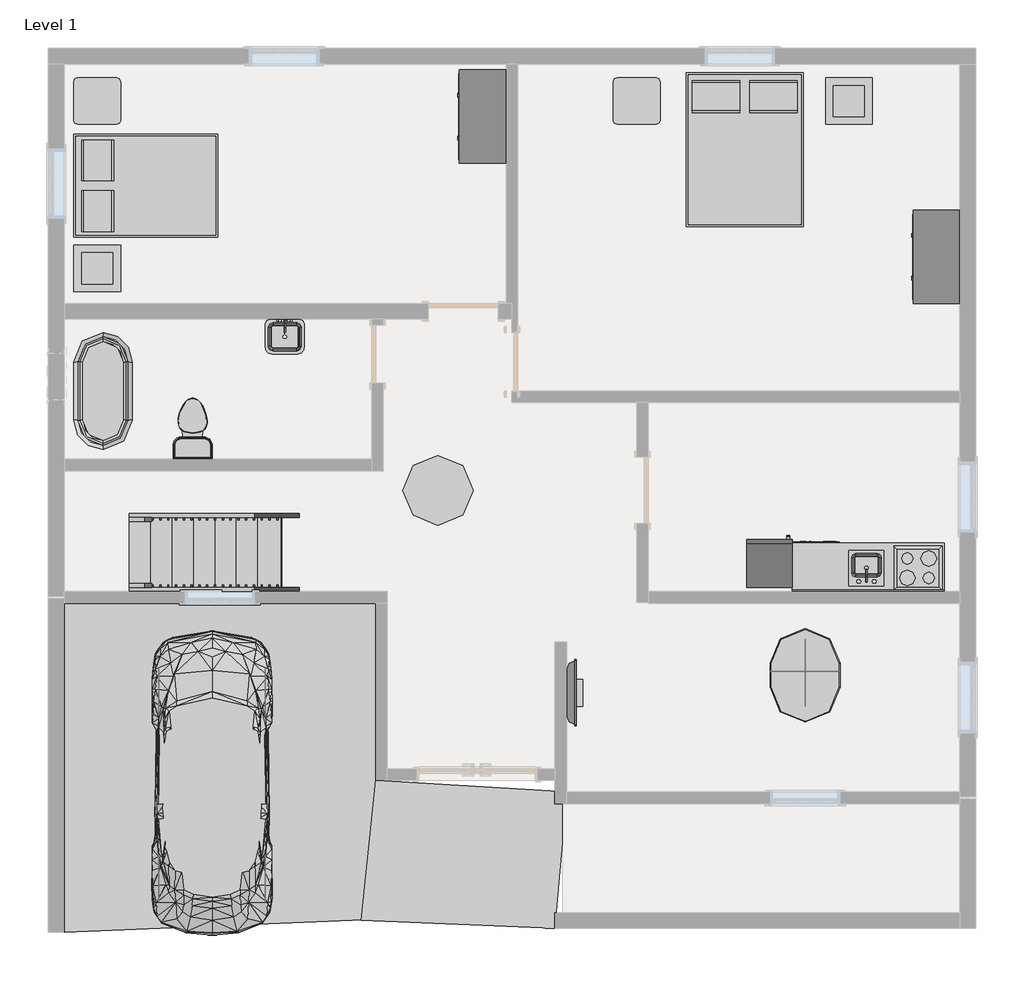
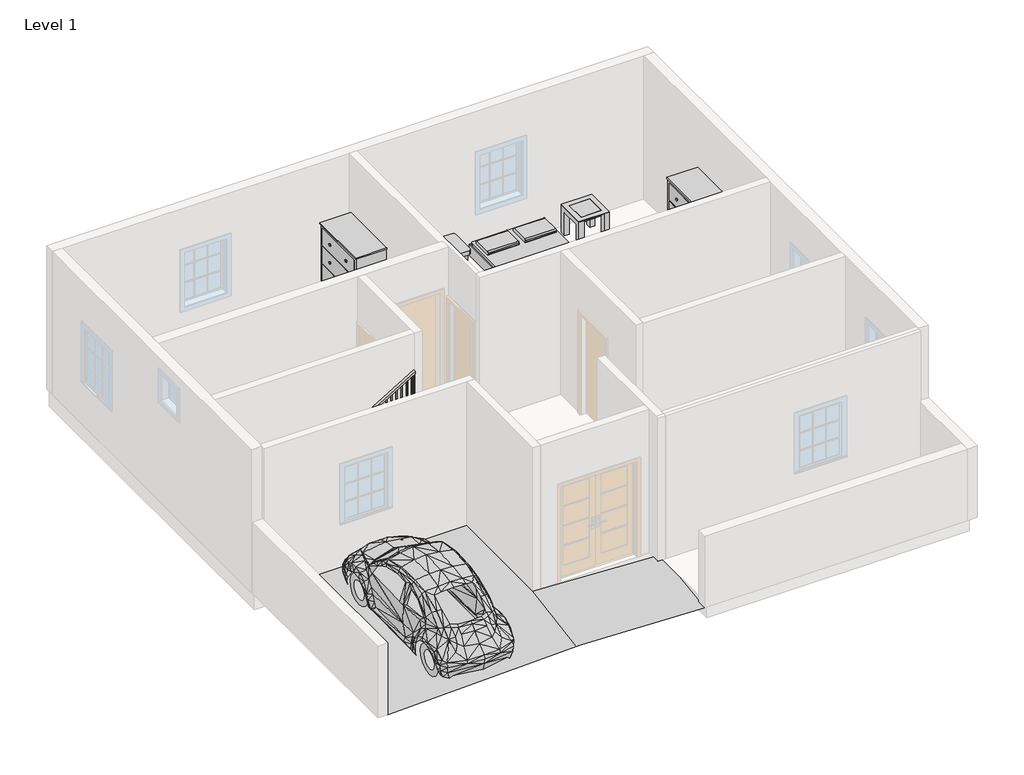
# One storey, part 2 of 2: 12 furniture elements, 7 proxies, 5 flow terminals, 2 members, 2 railings, 1 geographic element, 1 stair flight.
"""IFC4 building model written with IfcOpenShell, lengths in millimetres."""

from ifc_helpers import new_model, si_unit, frame, origin, place, context, project, spatial, polyline, outline, extrude, triangles, transform, mapped, element, save
from components import proxy_a6faaae8, proxy_45b28599, kitchenette_medium_kitchenette_medium_844211aa, rpc_beetle_rpc_beetle_3ce7ba48, proxy_c523a7b7, flow_terminal_2b63360b, flow_terminal_871c2e40, flow_terminal_62a433f7, toilet_domestic_3d_toilet_domestic_3d_f7549cf7, toilet_domestic_3d_toilet_domestic_3d_183bbd19, flow_terminal_b374fae2, furniture_c8abb964, furniture_1d2926bd, furniture_c6510c7c, furniture_9fa109b2, furniture_56245f3a, furniture_b5c51a22, furniture_be1c6672, furniture_905aceb5, furniture_bcf351fa, rpc_plant_tropical_agave_1_5_93a2a214, stair_flight_ef839ef7

model = new_model("IFC4")

# Units and contexts
model_context = context("Model", 3, world=origin())
ifc_project = project(units=[si_unit("LENGTHUNIT", "METRE", prefix="MILLI")], contexts=[model_context])

# Site, building, storey
site = spatial("IfcSite", under=ifc_project)
building = spatial("IfcBuilding", under=site)
storey = spatial("IfcBuildingStorey", under=building, Name="Level 1", Elevation=0.0)

# Proxies
placement = place(None, origin())
element("IfcBuildingElementProxy", 1, Name="Building Element Proxy", at=placement, inside=storey, context=model_context, shape_type="Tessellation", body=[
    triangles([(-9823.2573761, 4081.3729706, 0.0), (-7334.0575699, 3928.9729706, 0.0), (-7486.4575699, 2150.9729221, 0.0), (-9704.2471985, 2259.3859268, 0.0), (-10012.857431, 2253.2262737, 0.0)], [[1, 5, 4], [4, 3, 2], [3, 4, 5], [4, 2, 1]], closed=False),
])
element("IfcBuildingElementProxy", 2, Name="Building Element Proxy", at=placement, inside=storey, context=model_context, shape_type="Tessellation", body=[
    triangles([(-13887.2581512, 6392.7731644, 0.0), (-13887.2581512, 2100.1729706, 0.0), (-9823.2573761, 6392.7731644, 0.0), (-9969.6902985, 2259.3859268, 0.0), (-9823.2573761, 4081.3729706, 0.0)], [[1, 2, 5], [5, 3, 1], [5, 2, 4]], closed=False),
])
proxy_shape = proxy_a6faaae8(model_context)
element("IfcBuildingElementProxy", 3, Name="Cook Top-4 Unit2 : 22\" x 20\"", ObjectType="Cook Top-4 Unit2 : 22\" x 20\"", at=placement, inside=storey, context=model_context, shape_type="MappedRepresentation", body=[
    mapped(proxy_shape, transform((-2749.3576657, 6849.9729822, 0.0), x_axis=(-0.9999999999999998, 0.0, 0.0), y_axis=(0.0, -0.9999999999999998, 0.0), z_axis=(0.0, 0.0, 1.0))),
])
proxy_2_shape = proxy_45b28599(model_context)
element("IfcBuildingElementProxy", 4, Name="Dishwasher : 24\" x 24\" x 34\"", ObjectType="Dishwasher : 24\" x 24\" x 34\"", at=placement, inside=storey, context=model_context, shape_type="MappedRepresentation", body=[
    mapped(proxy_2_shape, transform((-3700.5401972, 7141.822547, 0.0), x_axis=(-0.9999999999999998, 0.0, 0.0), y_axis=(0.0, -0.9999999999999998, 0.0), z_axis=(0.0, 0.0, 1.0))),
])
kitchenette_medium_kitchenette_medium_shape = kitchenette_medium_kitchenette_medium_844211aa(model_context)
element("IfcBuildingElementProxy", 5, Name="Kitchenette - Medium : Kitchenette - Medium", ObjectType="Kitchenette - Medium : Kitchenette - Medium", at=placement, inside=storey, context=model_context, shape_type="MappedRepresentation", body=[
    mapped(kitchenette_medium_kitchenette_medium_shape, transform((-3073.5199608, 6545.1729822, 0.0), x_axis=(-0.9999999999999998, 0.0, 0.0), y_axis=(0.0, -0.9999999999999998, 0.0), z_axis=(0.0, 0.0, 1.0))),
])
rpc_beetle_rpc_beetle_shape = rpc_beetle_rpc_beetle_3ce7ba48(model_context)
element("IfcBuildingElementProxy", 6, Name="RPC Beetle : RPC Beetle", ObjectType="RPC Beetle : RPC Beetle", at=placement, inside=storey, context=model_context, shape_type="MappedRepresentation", body=[
    mapped(rpc_beetle_rpc_beetle_shape, transform((-11956.8576657, 2811.3729822, 0.0), x_axis=(1.0, 0.0, 0.0), y_axis=(0.0, 1.0, 0.0), z_axis=(0.0, 0.0, 1.0))),
])
proxy_3_shape = proxy_c523a7b7(model_context)
element("IfcBuildingElementProxy", 7, Name="Refrigerator : 24\" x 25\" LH", ObjectType="Refrigerator : 24\" x 25\" LH", at=placement, inside=storey, context=model_context, shape_type="MappedRepresentation", body=[
    mapped(proxy_3_shape, transform((-4686.1076657, 6895.6219537, 0.0), x_axis=(-0.9999999999999998, 0.0, 0.0), y_axis=(0.0, -0.9999999999999998, 0.0), z_axis=(0.0, 0.0, 1.0))),
])

# Flow terminals
flow_terminal_shape = flow_terminal_2b63360b(model_context)
element("IfcFlowTerminal", 8, ObjectType="Floor Drain - Rectangular : 5\"x5\" Strainer - 2\" Drain", at=placement, inside=storey, context=model_context, shape_type="MappedRepresentation", body=[
    mapped(flow_terminal_shape, transform((-12642.6576657, 9770.9729822, 0.0), x_axis=(1.0, 0.0, 0.0), y_axis=(0.0, 1.0, 0.0), z_axis=(0.0, 0.0, 1.0))),
])
flow_terminal_2_shape = flow_terminal_871c2e40(model_context)
element("IfcFlowTerminal", 9, ObjectType="Sink Kitchen-Island : 18\" x 18\"", at=placement, inside=storey, context=model_context, shape_type="MappedRepresentation", body=[
    mapped(flow_terminal_2_shape, transform((-3406.7684252, 6852.3183833, -14.4), x_axis=(-0.9999999999999998, 0.0, 0.0), y_axis=(0.0, -0.9999999999999998, 0.0), z_axis=(0.0, 0.0, 1.0))),
])
flow_terminal_3_shape = flow_terminal_62a433f7(model_context)
element("IfcFlowTerminal", 10, ObjectType="Sink Vanity-Square : 20\" x 18\"", at=placement, inside=storey, context=model_context, shape_type="MappedRepresentation", body=[
    mapped(flow_terminal_3_shape, transform((-11023.3628721, 9921.0275811, 0.0), x_axis=(1.0, 0.0, 0.0), y_axis=(0.0, 1.0, 0.0), z_axis=(0.0, 0.0, 1.0))),
])
toilet_domestic_3d_toilet_domestic_3d_shape = toilet_domestic_3d_toilet_domestic_3d_f7549cf7(model_context)
toilet_domestic_3d_toilet_domestic_3d_2_shape = toilet_domestic_3d_toilet_domestic_3d_183bbd19(model_context)
element("IfcFlowTerminal", 11, ObjectType="Toilet-Domestic-3D : Toilet-Domestic-3D", at=placement, inside=storey, context=model_context, shape_type="MappedRepresentation", body=[
    mapped(toilet_domestic_3d_toilet_domestic_3d_shape, transform((-12210.8576657, 8767.0690096, 0.0), x_axis=(-0.9999999999999998, 0.0, 0.0), y_axis=(0.0, -0.9999999999999998, 0.0), z_axis=(0.0, 0.0, 1.0))),
    mapped(toilet_domestic_3d_toilet_domestic_3d_2_shape, transform((-12210.8576657, 8767.0690096, 0.0), x_axis=(-0.9999999999999998, 0.0, 0.0), y_axis=(0.0, -0.9999999999999998, 0.0), z_axis=(0.0, 0.0, 1.0))),
])
flow_terminal_4_shape = flow_terminal_b374fae2(model_context)
element("IfcFlowTerminal", 12, ObjectType="Tub-Free Standing-3D : 30\" x 60\"", at=placement, inside=storey, context=model_context, shape_type="MappedRepresentation", body=[
    mapped(flow_terminal_4_shape, transform((-13379.2576657, 9161.3729822, 0.0), x_axis=(1.0, 0.0, 0.0), y_axis=(0.0, 1.0, 0.0), z_axis=(0.0, 0.0, 1.0))),
])

# Furniture
furniture_shape = furniture_c8abb964(model_context)
element("IfcFurniture", 13, ObjectType="Bed-Box : Double 53\" x 74\"", at=placement, inside=storey, context=model_context, shape_type="MappedRepresentation", body=[
    mapped(furniture_shape, transform((-13054.8871739, 11501.9205232, 0.0), x_axis=(0.0, 1.0, 0.0), y_axis=(-1.0, 0.0, 0.0), z_axis=(0.0, 0.0, 1.0))),
])
furniture_2_shape = furniture_1d2926bd(model_context)
element("IfcFurniture", 14, ObjectType="Bed-Box : Queen 60\" x 79\"", at=placement, inside=storey, context=model_context, shape_type="MappedRepresentation", body=[
    mapped(furniture_2_shape, transform((-5349.1101248, 12545.4024904, 0.0), x_axis=(1.0, 0.0, 0.0), y_axis=(0.0, 1.0, 0.0), z_axis=(0.0, 0.0, 1.0))),
])
furniture_3_shape = furniture_c6510c7c(model_context)
element("IfcFurniture", 15, ObjectType="Counter Top w Sink Hole : 24\" Depth", at=placement, inside=storey, context=model_context, shape_type="MappedRepresentation", body=[
    mapped(furniture_3_shape, transform((-3606.9199608, 6545.1729822, -14.4), x_axis=(-0.9999999999999998, 0.0, 0.0), y_axis=(0.0, -0.9999999999999998, 0.0), z_axis=(0.0, 0.0, 1.0))),
])
furniture_4_shape = furniture_9fa109b2(model_context)
element("IfcFurniture", 16, ObjectType="Dresser : 48\" x 72\" x 24\"", at=placement, inside=storey, context=model_context, shape_type="MappedRepresentation", body=[
    mapped(furniture_4_shape, transform((-8063.0947116, 12473.5797224, 0.0), x_axis=(0.0, -1.0000000000000007, 0.0), y_axis=(1.0000000000000007, 0.0, 0.0), z_axis=(0.0, 0.0, 1.0))),
])
element("IfcFurniture", 17, ObjectType="Dresser : 48\" x 72\" x 24\"", at=placement, inside=storey, context=model_context, shape_type="MappedRepresentation", body=[
    mapped(furniture_4_shape, transform((-2144.8947116, 10644.7797224, 0.0), x_axis=(0.0, -1.0000000000000007, 0.0), y_axis=(1.0000000000000007, 0.0, 0.0), z_axis=(0.0, 0.0, 1.0))),
])
furniture_5_shape = furniture_56245f3a(model_context)
element("IfcFurniture", 18, ObjectType="TV - Flat Screen : 32\"", at=placement, inside=storey, context=model_context, shape_type="MappedRepresentation", body=[
    mapped(furniture_5_shape, transform((-7275.5190421, 5228.3174964, 914.4), x_axis=(0.0, 1.0, 0.0), y_axis=(-1.0, 0.0, 0.0), z_axis=(0.0, 0.0, 1.0))),
])
furniture_6_shape = furniture_b5c51a22(model_context)
element("IfcFurniture", 19, ObjectType="Table-Coffee : 24\" x 24\" x 24\"", at=placement, inside=storey, context=model_context, shape_type="MappedRepresentation", body=[
    mapped(furniture_6_shape, transform((-13473.7234324, 10666.3619044, 0.0), x_axis=(1.0, 0.0, 0.0), y_axis=(0.0, 1.0, 0.0), z_axis=(0.0, 0.0, 1.0))),
])
element("IfcFurniture", 20, ObjectType="Table-Coffee : 24\" x 24\" x 24\"", at=placement, inside=storey, context=model_context, shape_type="MappedRepresentation", body=[
    mapped(furniture_6_shape, transform((-3669.3234324, 12850.7619044, 0.0), x_axis=(1.0, 0.0, 0.0), y_axis=(0.0, 1.0, 0.0), z_axis=(0.0, 0.0, 1.0))),
])
furniture_7_shape = furniture_be1c6672(model_context)
element("IfcFurniture", 21, ObjectType="Table-Dining Oval : 36\" x 48\"", at=placement, inside=storey, context=model_context, shape_type="MappedRepresentation", body=[
    mapped(furniture_7_shape, transform((-4580.6560264, 5854.7926544, 0.0), x_axis=(0.0, 1.0000000000000002, 0.0), y_axis=(-1.0000000000000002, 0.0, 0.0), z_axis=(0.0, 0.0, 1.0))),
])
furniture_8_shape = furniture_905aceb5(model_context)
element("IfcFurniture", 22, ObjectType="Table-Dining Round w Chairs : 36\" Diameter", at=placement, inside=storey, context=model_context, shape_type="MappedRepresentation", body=[
    mapped(furniture_8_shape, transform((-9114.139633, 8050.8516707, 0.0), x_axis=(1.0, 0.0, 0.0), y_axis=(0.0, 1.0, 0.0), z_axis=(0.0, 0.0, 1.0))),
])
furniture_9_shape = furniture_bcf351fa(model_context)
element("IfcFurniture", 23, ObjectType="Table-End : 24\" x 24\"", at=placement, inside=storey, context=model_context, shape_type="MappedRepresentation", body=[
    mapped(furniture_9_shape, transform((-13763.991296, 12793.5729822, 0.0), x_axis=(1.0, 0.0, 0.0), y_axis=(0.0, 1.0, 0.0), z_axis=(0.0, 0.0, 1.0))),
])
element("IfcFurniture", 24, ObjectType="Table-End : 24\" x 24\"", at=placement, inside=storey, context=model_context, shape_type="MappedRepresentation", body=[
    mapped(furniture_9_shape, transform((-6728.191296, 12793.5729822, 0.0), x_axis=(1.0, 0.0, 0.0), y_axis=(0.0, 1.0, 0.0), z_axis=(0.0, 0.0, 1.0))),
])

# Geographic element
rpc_plant_tropical_agave_1_5_shape = rpc_plant_tropical_agave_1_5_93a2a214(model_context)
element("IfcGeographicElement", 25, ObjectType="RPC Plant - Tropical : Agave - 1.5'", at=placement, inside=storey, context=model_context, shape_type="MappedRepresentation", body=[
    mapped(rpc_plant_tropical_agave_1_5_shape, transform((-4222.5576657, 5503.7729822, 609.6), x_axis=(1.0, 0.0, 0.0), y_axis=(0.0, 1.0, 0.0), z_axis=(0.0, 0.0, 1.0))),
])

# Members
element("IfcMember", 26, ObjectType="Stringer - 2\" Width", at=placement, inside=storey, context=model_context, shape_type="SweptSolid", body=[
    extrude(outline(polyline([(212.114512, -13036.36961), (0.0, -13036.36961), (0.0, -12798.2840982), (1549.0390838, -10242.36961), (1905.4478453, -10242.36961), (212.114512, -13036.36961)])), frame((0.0, 7512.7146616, 0.0), z_axis=(0.0, 1.0, 0.0), x_axis=(0.0, 0.0, 1.0)), (0.0, 0.0, 1.0), 50.8),
])
element("IfcMember", 27, ObjectType="Stringer - 2\" Width", at=placement, inside=storey, context=model_context, shape_type="SweptSolid", body=[
    extrude(outline(polyline([(212.114512, -13036.36961), (0.0, -13036.36961), (0.0, -12798.2840982), (1549.0390838, -10242.36961), (1905.4478453, -10242.36961), (212.114512, -13036.36961)])), frame((0.0, 6547.5146616, 0.0), z_axis=(0.0, 1.0, 0.0), x_axis=(0.0, 0.0, 1.0)), (0.0, 0.0, 1.0), 50.8),
])

# Railings
element("IfcRailing", 28, ObjectType="Handrail - Rectangular", at=placement, inside=storey, context=model_context, shape_type="SweptSolid", body=[
    extrude(outline(polyline([(1083.7333333, -13036.36961), (1024.3318731, -13036.36961), (2717.6652064, -10242.36961), (2777.0666667, -10242.36961), (1083.7333333, -13036.36961)])), frame((0.0, 6598.3146616, 0.0), z_axis=(0.0, 1.0, 0.0), x_axis=(0.0, 0.0, 1.0)), (0.0, 0.0, 1.0), 50.8),
    extrude(outline(polyline([(2692.6500549, -10283.64461), (2681.1046004, -10302.69461), (1693.3333333, -10302.69461), (1693.3333333, -10283.64461), (2692.6500549, -10283.64461)])), frame((0.0, 6614.1896616, 0.0), z_axis=(0.0, 1.0, 0.0), x_axis=(0.0, 0.0, 1.0)), (0.0, 0.0, 1.0), 19.05),
    extrude(outline(polyline([(2631.0742973, -10385.24461), (2619.5288428, -10404.29461), (1693.3333333, -10404.29461), (1693.3333333, -10385.24461), (2631.0742973, -10385.24461)])), frame((0.0, 6614.1896616, 0.0), z_axis=(0.0, 1.0, 0.0), x_axis=(0.0, 0.0, 1.0)), (0.0, 0.0, 1.0), 19.05),
    extrude(outline(polyline([(2569.4985397, -10486.84461), (2557.9530852, -10505.89461), (1693.3333333, -10505.89461), (1693.3333333, -10486.84461), (2569.4985397, -10486.84461)])), frame((0.0, 6614.1896616, 0.0), z_axis=(0.0, 1.0, 0.0), x_axis=(0.0, 0.0, 1.0)), (0.0, 0.0, 1.0), 19.05),
    extrude(outline(polyline([(2507.9227822, -10588.44461), (2496.3773276, -10607.49461), (1524.0, -10607.49461), (1524.0, -10588.44461), (2507.9227822, -10588.44461)])), frame((0.0, 6614.1896616, 0.0), z_axis=(0.0, 1.0, 0.0), x_axis=(0.0, 0.0, 1.0)), (0.0, 0.0, 1.0), 19.05),
    extrude(outline(polyline([(2446.3470246, -10690.04461), (2434.80157, -10709.09461), (1524.0, -10709.09461), (1524.0, -10690.04461), (2446.3470246, -10690.04461)])), frame((0.0, 6614.1896616, 0.0), z_axis=(0.0, 1.0, 0.0), x_axis=(0.0, 0.0, 1.0)), (0.0, 0.0, 1.0), 19.05),
    extrude(outline(polyline([(2384.771267, -10791.64461), (2373.2258125, -10810.69461), (1524.0, -10810.69461), (1524.0, -10791.64461), (2384.771267, -10791.64461)])), frame((0.0, 6614.1896616, 0.0), z_axis=(0.0, 1.0, 0.0), x_axis=(0.0, 0.0, 1.0)), (0.0, 0.0, 1.0), 19.05),
    extrude(outline(polyline([(2323.1955094, -10893.24461), (2311.6500549, -10912.29461), (1354.6666667, -10912.29461), (1354.6666667, -10893.24461), (2323.1955094, -10893.24461)])), frame((0.0, 6614.1896616, 0.0), z_axis=(0.0, 1.0, 0.0), x_axis=(0.0, 0.0, 1.0)), (0.0, 0.0, 1.0), 19.05),
    extrude(outline(polyline([(2261.6197519, -10994.84461), (2250.0742973, -11013.89461), (1354.6666667, -11013.89461), (1354.6666667, -10994.84461), (2261.6197519, -10994.84461)])), frame((0.0, 6614.1896616, 0.0), z_axis=(0.0, 1.0, 0.0), x_axis=(0.0, 0.0, 1.0)), (0.0, 0.0, 1.0), 19.05),
    extrude(outline(polyline([(2200.0439943, -11096.44461), (2188.4985397, -11115.49461), (1185.3333333, -11115.49461), (1185.3333333, -11096.44461), (2200.0439943, -11096.44461)])), frame((0.0, 6614.1896616, 0.0), z_axis=(0.0, 1.0, 0.0), x_axis=(0.0, 0.0, 1.0)), (0.0, 0.0, 1.0), 19.05),
    extrude(outline(polyline([(2138.4682367, -11198.04461), (2126.9227822, -11217.09461), (1185.3333333, -11217.09461), (1185.3333333, -11198.04461), (2138.4682367, -11198.04461)])), frame((0.0, 6614.1896616, 0.0), z_axis=(0.0, 1.0, 0.0), x_axis=(0.0, 0.0, 1.0)), (0.0, 0.0, 1.0), 19.05),
    extrude(outline(polyline([(2076.8924791, -11299.64461), (2065.3470246, -11318.69461), (1185.3333333, -11318.69461), (1185.3333333, -11299.64461), (2076.8924791, -11299.64461)])), frame((0.0, 6614.1896616, 0.0), z_axis=(0.0, 1.0, 0.0), x_axis=(0.0, 0.0, 1.0)), (0.0, 0.0, 1.0), 19.05),
    extrude(outline(polyline([(2015.3167216, -11401.24461), (2003.771267, -11420.29461), (1016.0, -11420.29461), (1016.0, -11401.24461), (2015.3167216, -11401.24461)])), frame((0.0, 6614.1896616, 0.0), z_axis=(0.0, 1.0, 0.0), x_axis=(0.0, 0.0, 1.0)), (0.0, 0.0, 1.0), 19.05),
    extrude(outline(polyline([(1953.740964, -11502.84461), (1942.1955094, -11521.89461), (1016.0, -11521.89461), (1016.0, -11502.84461), (1953.740964, -11502.84461)])), frame((0.0, 6614.1896616, 0.0), z_axis=(0.0, 1.0, 0.0), x_axis=(0.0, 0.0, 1.0)), (0.0, 0.0, 1.0), 19.05),
    extrude(outline(polyline([(1892.1652064, -11604.44461), (1880.6197519, -11623.49461), (1016.0, -11623.49461), (1016.0, -11604.44461), (1892.1652064, -11604.44461)])), frame((0.0, 6614.1896616, 0.0), z_axis=(0.0, 1.0, 0.0), x_axis=(0.0, 0.0, 1.0)), (0.0, 0.0, 1.0), 19.05),
    extrude(outline(polyline([(1830.5894488, -11706.04461), (1819.0439943, -11725.09461), (846.6666667, -11725.09461), (846.6666667, -11706.04461), (1830.5894488, -11706.04461)])), frame((0.0, 6614.1896616, 0.0), z_axis=(0.0, 1.0, 0.0), x_axis=(0.0, 0.0, 1.0)), (0.0, 0.0, 1.0), 19.05),
    extrude(outline(polyline([(1769.0136913, -11807.64461), (1757.4682367, -11826.69461), (846.6666667, -11826.69461), (846.6666667, -11807.64461), (1769.0136913, -11807.64461)])), frame((0.0, 6614.1896616, 0.0), z_axis=(0.0, 1.0, 0.0), x_axis=(0.0, 0.0, 1.0)), (0.0, 0.0, 1.0), 19.05),
    extrude(outline(polyline([(1707.4379337, -11909.24461), (1695.8924791, -11928.29461), (846.6666667, -11928.29461), (846.6666667, -11909.24461), (1707.4379337, -11909.24461)])), frame((0.0, 6614.1896616, 0.0), z_axis=(0.0, 1.0, 0.0), x_axis=(0.0, 0.0, 1.0)), (0.0, 0.0, 1.0), 19.05),
    extrude(outline(polyline([(1645.8621761, -12010.84461), (1634.3167216, -12029.89461), (677.3333333, -12029.89461), (677.3333333, -12010.84461), (1645.8621761, -12010.84461)])), frame((0.0, 6614.1896616, 0.0), z_axis=(0.0, 1.0, 0.0), x_axis=(0.0, 0.0, 1.0)), (0.0, 0.0, 1.0), 19.05),
    extrude(outline(polyline([(1584.2864185, -12112.44461), (1572.740964, -12131.49461), (677.3333333, -12131.49461), (677.3333333, -12112.44461), (1584.2864185, -12112.44461)])), frame((0.0, 6614.1896616, 0.0), z_axis=(0.0, 1.0, 0.0), x_axis=(0.0, 0.0, 1.0)), (0.0, 0.0, 1.0), 19.05),
    extrude(outline(polyline([(1522.710661, -12214.04461), (1511.1652064, -12233.09461), (508.0, -12233.09461), (508.0, -12214.04461), (1522.710661, -12214.04461)])), frame((0.0, 6614.1896616, 0.0), z_axis=(0.0, 1.0, 0.0), x_axis=(0.0, 0.0, 1.0)), (0.0, 0.0, 1.0), 19.05),
    extrude(outline(polyline([(1461.1349034, -12315.64461), (1449.5894488, -12334.69461), (508.0, -12334.69461), (508.0, -12315.64461), (1461.1349034, -12315.64461)])), frame((0.0, 6614.1896616, 0.0), z_axis=(0.0, 1.0, 0.0), x_axis=(0.0, 0.0, 1.0)), (0.0, 0.0, 1.0), 19.05),
    extrude(outline(polyline([(1399.5591458, -12417.24461), (1388.0136913, -12436.29461), (508.0, -12436.29461), (508.0, -12417.24461), (1399.5591458, -12417.24461)])), frame((0.0, 6614.1896616, 0.0), z_axis=(0.0, 1.0, 0.0), x_axis=(0.0, 0.0, 1.0)), (0.0, 0.0, 1.0), 19.05),
    extrude(outline(polyline([(1337.9833882, -12518.84461), (1326.4379337, -12537.89461), (338.6666667, -12537.89461), (338.6666667, -12518.84461), (1337.9833882, -12518.84461)])), frame((0.0, 6614.1896616, 0.0), z_axis=(0.0, 1.0, 0.0), x_axis=(0.0, 0.0, 1.0)), (0.0, 0.0, 1.0), 19.05),
    extrude(outline(polyline([(1276.4076307, -12620.44461), (1264.8621761, -12639.49461), (338.6666667, -12639.49461), (338.6666667, -12620.44461), (1276.4076307, -12620.44461)])), frame((0.0, 6614.1896616, 0.0), z_axis=(0.0, 1.0, 0.0), x_axis=(0.0, 0.0, 1.0)), (0.0, 0.0, 1.0), 19.05),
    extrude(outline(polyline([(1214.8318731, -12722.04461), (1203.2864185, -12741.09461), (338.6666667, -12741.09461), (338.6666667, -12722.04461), (1214.8318731, -12722.04461)])), frame((0.0, 6614.1896616, 0.0), z_axis=(0.0, 1.0, 0.0), x_axis=(0.0, 0.0, 1.0)), (0.0, 0.0, 1.0), 19.05),
    extrude(outline(polyline([(1153.2561155, -12823.64461), (1141.710661, -12842.69461), (169.3333333, -12842.69461), (169.3333333, -12823.64461), (1153.2561155, -12823.64461)])), frame((0.0, 6614.1896616, 0.0), z_axis=(0.0, 1.0, 0.0), x_axis=(0.0, 0.0, 1.0)), (0.0, 0.0, 1.0), 19.05),
    extrude(outline(polyline([(1091.6803579, -12925.24461), (1080.1349034, -12944.29461), (169.3333333, -12944.29461), (169.3333333, -12925.24461), (1091.6803579, -12925.24461)])), frame((0.0, 6614.1896616, 0.0), z_axis=(0.0, 1.0, 0.0), x_axis=(0.0, 0.0, 1.0)), (0.0, 0.0, 1.0), 19.05),
    extrude(outline(polyline([(2717.6652064, -10242.36961), (2706.1197519, -10261.41961), (1693.3333333, -10261.41961), (1693.3333333, -10242.36961), (2717.6652064, -10242.36961)])), frame((0.0, 6614.1896616, 0.0), z_axis=(0.0, 1.0, 0.0), x_axis=(0.0, 0.0, 1.0)), (0.0, 0.0, 1.0), 19.05),
    extrude(outline(polyline([(1035.8773276, -13017.31961), (1024.3318731, -13036.36961), (169.3333333, -13036.36961), (169.3333333, -13017.31961), (1035.8773276, -13017.31961)])), frame((0.0, 6614.1896616, 0.0), z_axis=(0.0, 1.0, 0.0), x_axis=(0.0, 0.0, 1.0)), (0.0, 0.0, 1.0), 19.05),
])
element("IfcRailing", 29, ObjectType="Handrail - Rectangular", at=placement, inside=storey, context=model_context, shape_type="SweptSolid", body=[
    extrude(outline(polyline([(1083.7333333, -13036.36961), (1024.3318731, -13036.36961), (2717.6652064, -10242.36961), (2777.0666667, -10242.36961), (1083.7333333, -13036.36961)])), frame((0.0, 7461.9146616, 0.0), z_axis=(0.0, 1.0, 0.0), x_axis=(0.0, 0.0, 1.0)), (0.0, 0.0, 1.0), 50.8),
    extrude(outline(polyline([(2681.1046004, -10302.69461), (1693.3333333, -10302.69461), (1693.3333333, -10283.64461), (2692.6500549, -10283.64461), (2681.1046004, -10302.69461)])), frame((0.0, 7477.7896616, 0.0), z_axis=(0.0, 1.0, 0.0), x_axis=(0.0, 0.0, 1.0)), (0.0, 0.0, 1.0), 19.05),
    extrude(outline(polyline([(2619.5288428, -10404.29461), (1693.3333333, -10404.29461), (1693.3333333, -10385.24461), (2631.0742973, -10385.24461), (2619.5288428, -10404.29461)])), frame((0.0, 7477.7896616, 0.0), z_axis=(0.0, 1.0, 0.0), x_axis=(0.0, 0.0, 1.0)), (0.0, 0.0, 1.0), 19.05),
    extrude(outline(polyline([(2557.9530852, -10505.89461), (1693.3333333, -10505.89461), (1693.3333333, -10486.84461), (2569.4985397, -10486.84461), (2557.9530852, -10505.89461)])), frame((0.0, 7477.7896616, 0.0), z_axis=(0.0, 1.0, 0.0), x_axis=(0.0, 0.0, 1.0)), (0.0, 0.0, 1.0), 19.05),
    extrude(outline(polyline([(2496.3773276, -10607.49461), (1524.0, -10607.49461), (1524.0, -10588.44461), (2507.9227822, -10588.44461), (2496.3773276, -10607.49461)])), frame((0.0, 7477.7896616, 0.0), z_axis=(0.0, 1.0, 0.0), x_axis=(0.0, 0.0, 1.0)), (0.0, 0.0, 1.0), 19.05),
    extrude(outline(polyline([(2434.80157, -10709.09461), (1524.0, -10709.09461), (1524.0, -10690.04461), (2446.3470246, -10690.04461), (2434.80157, -10709.09461)])), frame((0.0, 7477.7896616, 0.0), z_axis=(0.0, 1.0, 0.0), x_axis=(0.0, 0.0, 1.0)), (0.0, 0.0, 1.0), 19.05),
    extrude(outline(polyline([(2373.2258125, -10810.69461), (1524.0, -10810.69461), (1524.0, -10791.64461), (2384.771267, -10791.64461), (2373.2258125, -10810.69461)])), frame((0.0, 7477.7896616, 0.0), z_axis=(0.0, 1.0, 0.0), x_axis=(0.0, 0.0, 1.0)), (0.0, 0.0, 1.0), 19.05),
    extrude(outline(polyline([(2311.6500549, -10912.29461), (1354.6666667, -10912.29461), (1354.6666667, -10893.24461), (2323.1955094, -10893.24461), (2311.6500549, -10912.29461)])), frame((0.0, 7477.7896616, 0.0), z_axis=(0.0, 1.0, 0.0), x_axis=(0.0, 0.0, 1.0)), (0.0, 0.0, 1.0), 19.05),
    extrude(outline(polyline([(2250.0742973, -11013.89461), (1354.6666667, -11013.89461), (1354.6666667, -10994.84461), (2261.6197519, -10994.84461), (2250.0742973, -11013.89461)])), frame((0.0, 7477.7896616, 0.0), z_axis=(0.0, 1.0, 0.0), x_axis=(0.0, 0.0, 1.0)), (0.0, 0.0, 1.0), 19.05),
    extrude(outline(polyline([(2188.4985397, -11115.49461), (1185.3333333, -11115.49461), (1185.3333333, -11096.44461), (2200.0439943, -11096.44461), (2188.4985397, -11115.49461)])), frame((0.0, 7477.7896616, 0.0), z_axis=(0.0, 1.0, 0.0), x_axis=(0.0, 0.0, 1.0)), (0.0, 0.0, 1.0), 19.05),
    extrude(outline(polyline([(2126.9227822, -11217.09461), (1185.3333333, -11217.09461), (1185.3333333, -11198.04461), (2138.4682367, -11198.04461), (2126.9227822, -11217.09461)])), frame((0.0, 7477.7896616, 0.0), z_axis=(0.0, 1.0, 0.0), x_axis=(0.0, 0.0, 1.0)), (0.0, 0.0, 1.0), 19.05),
    extrude(outline(polyline([(2065.3470246, -11318.69461), (1185.3333333, -11318.69461), (1185.3333333, -11299.64461), (2076.8924791, -11299.64461), (2065.3470246, -11318.69461)])), frame((0.0, 7477.7896616, 0.0), z_axis=(0.0, 1.0, 0.0), x_axis=(0.0, 0.0, 1.0)), (0.0, 0.0, 1.0), 19.05),
    extrude(outline(polyline([(2003.771267, -11420.29461), (1016.0, -11420.29461), (1016.0, -11401.24461), (2015.3167216, -11401.24461), (2003.771267, -11420.29461)])), frame((0.0, 7477.7896616, 0.0), z_axis=(0.0, 1.0, 0.0), x_axis=(0.0, 0.0, 1.0)), (0.0, 0.0, 1.0), 19.05),
    extrude(outline(polyline([(1942.1955094, -11521.89461), (1016.0, -11521.89461), (1016.0, -11502.84461), (1953.740964, -11502.84461), (1942.1955094, -11521.89461)])), frame((0.0, 7477.7896616, 0.0), z_axis=(0.0, 1.0, 0.0), x_axis=(0.0, 0.0, 1.0)), (0.0, 0.0, 1.0), 19.05),
    extrude(outline(polyline([(1880.6197519, -11623.49461), (1016.0, -11623.49461), (1016.0, -11604.44461), (1892.1652064, -11604.44461), (1880.6197519, -11623.49461)])), frame((0.0, 7477.7896616, 0.0), z_axis=(0.0, 1.0, 0.0), x_axis=(0.0, 0.0, 1.0)), (0.0, 0.0, 1.0), 19.05),
    extrude(outline(polyline([(1819.0439943, -11725.09461), (846.6666667, -11725.09461), (846.6666667, -11706.04461), (1830.5894488, -11706.04461), (1819.0439943, -11725.09461)])), frame((0.0, 7477.7896616, 0.0), z_axis=(0.0, 1.0, 0.0), x_axis=(0.0, 0.0, 1.0)), (0.0, 0.0, 1.0), 19.05),
    extrude(outline(polyline([(1757.4682367, -11826.69461), (846.6666667, -11826.69461), (846.6666667, -11807.64461), (1769.0136913, -11807.64461), (1757.4682367, -11826.69461)])), frame((0.0, 7477.7896616, 0.0), z_axis=(0.0, 1.0, 0.0), x_axis=(0.0, 0.0, 1.0)), (0.0, 0.0, 1.0), 19.05),
    extrude(outline(polyline([(1695.8924791, -11928.29461), (846.6666667, -11928.29461), (846.6666667, -11909.24461), (1707.4379337, -11909.24461), (1695.8924791, -11928.29461)])), frame((0.0, 7477.7896616, 0.0), z_axis=(0.0, 1.0, 0.0), x_axis=(0.0, 0.0, 1.0)), (0.0, 0.0, 1.0), 19.05),
    extrude(outline(polyline([(1634.3167216, -12029.89461), (677.3333333, -12029.89461), (677.3333333, -12010.84461), (1645.8621761, -12010.84461), (1634.3167216, -12029.89461)])), frame((0.0, 7477.7896616, 0.0), z_axis=(0.0, 1.0, 0.0), x_axis=(0.0, 0.0, 1.0)), (0.0, 0.0, 1.0), 19.05),
    extrude(outline(polyline([(1572.740964, -12131.49461), (677.3333333, -12131.49461), (677.3333333, -12112.44461), (1584.2864185, -12112.44461), (1572.740964, -12131.49461)])), frame((0.0, 7477.7896616, 0.0), z_axis=(0.0, 1.0, 0.0), x_axis=(0.0, 0.0, 1.0)), (0.0, 0.0, 1.0), 19.05),
    extrude(outline(polyline([(1511.1652064, -12233.09461), (508.0, -12233.09461), (508.0, -12214.04461), (1522.710661, -12214.04461), (1511.1652064, -12233.09461)])), frame((0.0, 7477.7896616, 0.0), z_axis=(0.0, 1.0, 0.0), x_axis=(0.0, 0.0, 1.0)), (0.0, 0.0, 1.0), 19.05),
    extrude(outline(polyline([(1449.5894488, -12334.69461), (508.0, -12334.69461), (508.0, -12315.64461), (1461.1349034, -12315.64461), (1449.5894488, -12334.69461)])), frame((0.0, 7477.7896616, 0.0), z_axis=(0.0, 1.0, 0.0), x_axis=(0.0, 0.0, 1.0)), (0.0, 0.0, 1.0), 19.05),
    extrude(outline(polyline([(1388.0136913, -12436.29461), (508.0, -12436.29461), (508.0, -12417.24461), (1399.5591458, -12417.24461), (1388.0136913, -12436.29461)])), frame((0.0, 7477.7896616, 0.0), z_axis=(0.0, 1.0, 0.0), x_axis=(0.0, 0.0, 1.0)), (0.0, 0.0, 1.0), 19.05),
    extrude(outline(polyline([(1326.4379337, -12537.89461), (338.6666667, -12537.89461), (338.6666667, -12518.84461), (1337.9833882, -12518.84461), (1326.4379337, -12537.89461)])), frame((0.0, 7477.7896616, 0.0), z_axis=(0.0, 1.0, 0.0), x_axis=(0.0, 0.0, 1.0)), (0.0, 0.0, 1.0), 19.05),
    extrude(outline(polyline([(1264.8621761, -12639.49461), (338.6666667, -12639.49461), (338.6666667, -12620.44461), (1276.4076307, -12620.44461), (1264.8621761, -12639.49461)])), frame((0.0, 7477.7896616, 0.0), z_axis=(0.0, 1.0, 0.0), x_axis=(0.0, 0.0, 1.0)), (0.0, 0.0, 1.0), 19.05),
    extrude(outline(polyline([(1203.2864185, -12741.09461), (338.6666667, -12741.09461), (338.6666667, -12722.04461), (1214.8318731, -12722.04461), (1203.2864185, -12741.09461)])), frame((0.0, 7477.7896616, 0.0), z_axis=(0.0, 1.0, 0.0), x_axis=(0.0, 0.0, 1.0)), (0.0, 0.0, 1.0), 19.05),
    extrude(outline(polyline([(1141.710661, -12842.69461), (169.3333333, -12842.69461), (169.3333333, -12823.64461), (1153.2561155, -12823.64461), (1141.710661, -12842.69461)])), frame((0.0, 7477.7896616, 0.0), z_axis=(0.0, 1.0, 0.0), x_axis=(0.0, 0.0, 1.0)), (0.0, 0.0, 1.0), 19.05),
    extrude(outline(polyline([(1080.1349034, -12944.29461), (169.3333333, -12944.29461), (169.3333333, -12925.24461), (1091.6803579, -12925.24461), (1080.1349034, -12944.29461)])), frame((0.0, 7477.7896616, 0.0), z_axis=(0.0, 1.0, 0.0), x_axis=(0.0, 0.0, 1.0)), (0.0, 0.0, 1.0), 19.05),
    extrude(outline(polyline([(2706.1197519, -10261.41961), (1693.3333333, -10261.41961), (1693.3333333, -10242.36961), (2717.6652064, -10242.36961), (2706.1197519, -10261.41961)])), frame((0.0, 7477.7896616, 0.0), z_axis=(0.0, 1.0, 0.0), x_axis=(0.0, 0.0, 1.0)), (0.0, 0.0, 1.0), 19.05),
    extrude(outline(polyline([(1024.3318731, -13036.36961), (169.3333333, -13036.36961), (169.3333333, -13017.31961), (1035.8773276, -13017.31961), (1024.3318731, -13036.36961)])), frame((0.0, 7477.7896616, 0.0), z_axis=(0.0, 1.0, 0.0), x_axis=(0.0, 0.0, 1.0)), (0.0, 0.0, 1.0), 19.05),
])

# Stair flight
stair_flight_shape = stair_flight_ef839ef7(model_context)
element("IfcStairFlight", 30, ObjectType="2\" Tread 1\" Nosing 1/4\" Riser", at=placement, inside=storey, context=model_context, shape_type="MappedRepresentation", body=[
    mapped(stair_flight_shape, transform((0.0, 0.0, 0.0), x_axis=(1.0, 0.0, 0.0), y_axis=(0.0, 1.0, 0.0), z_axis=(0.0, 0.0, 1.0))),
])

save(model, "model.ifc")

# Revit data of these elements
# Type "Cook Top-4 Unit2 : 22\" x 20\""
#   Depth = 1' - 8"
#   Width = 1' - 10"
#   Burner Material = Steel, Chrome Plated
#   Cooktop Material = Steel, Polished
#   Default Elevation = 0
#   Assembly Code = ""
# Type "Dishwasher : 24\" x 24\" x 34\""
#   Label = "DW"
#   Assembly Code = "E1090400"
#   Depth = 2' - 0"
#   Height = 2' - 10"
#   Width = 2' - 0"
#   Dishwasher Material = Steel, Paint Finish, Ivory, Glossy
#   Panel Face Material = Plastic, Opaque Black
#   Default Elevation = 0
# Type "Kitchenette - Medium : Kitchenette - Medium"
#   Assembly Code = "E1090400"
#   Counter Length = 6' - 6"
#   Cabinet Width = 4' - 6"
#   Cabinet Height = 2' - 10 1/2"
#   Cabinet Depth = 2' - 0"
#   Toe Depth = 0' - 3"
#   Toe Height = 0' - 3 1/2"
#   Cabinet Material = Cabinets
#   Door/Drawer Material = Cabinets
#   Handle Material = Cabinets - Handles
#   Default Elevation = 0
# Type "RPC Beetle : RPC Beetle"
#   built-in parameter 1005195 = "RPC-16-0U6E-L4EG-ENH1-J3KF-SVEL-0TX4-C0"
#   Height = 0
# Type "Refrigerator : 24\" x 25\" LH"
#   Label = "REF."
#   Assembly Code = "E1090400"
#   Depth = 2' - 0 3/4"
#   Handle = 0' - 1 1/2"
#   Height = 5' - 3 1/2"
#   Rear Clearance = 0' - 2"
#   Top Door Height = 1' - 8"
#   Width = 1' - 11 1/2"
#   Material = Steel, Paint Finish, Ivory, Glossy
#   Default Elevation = 0
# Type "Floor Drain - Rectangular : 5\"x5\" Strainer - 2\" Drain"
#   WFU = 2
#   Strainer Height = 0' - 3 1/4"
#   Half Strainer Length = 0' - 2 1/2"
#   Strainer Length = 0' - 5"
#   Radius 2 = 0' - 3.04167"
#   Radius 1 = 0' - 2.02083"
#   Radius 3 = 0' - 2 1/32"
#   Pipe Radius = 1"
#   Pipe Diameter = 2"
#   Height 2 = 0' - 0.725"
#   Height 1 = 0' - 1 13/16"
#   Body Radius = 0' - 4 1/16"
#   Body Height = 0' - 3 5/8"
#   Body Diameter = 0' - 8 1/8"
#   Drain Material = none
#   HWFU = 0
#   Default Elevation = 0
#   CWFU = 0
# Type "Sink Kitchen-Island : 18\" x 18\""
#   Assembly Code = "D2010410"
#   Counter Height = 3' - 0"
#   Depth = 1' - 6"
#   Width = 1' - 6"
#   Faucet Material = Steel, Polished
#   Sink Material = Steel, Polished
#   Default Elevation = 0
# Type "Sink Vanity-Square : 20\" x 18\""
#   Assembly Code = "D2010400"
#   Counter Height = 2' - 7"
#   Depth = 1' - 6"
#   Width = 1' - 8"
#   Basin Material = Porcelain, Linen
#   Faucet Material = Steel, Polished
#   Default Elevation = 0
# Type "Toilet-Domestic-3D : Toilet-Domestic-3D"
#   Assembly Code = "D2010110"
#   Toilet - Bowl/Basin Material = Porcelain, Linen
#   Toilet - Seat Material = Laminate, Linen, Matte
#   Default Elevation = 0
# Type "Tub-Free Standing-3D : 30\" x 60\""
#   Assembly Code = "D2010110"
#   Height = 1' - 6"
#   Length = 5' - 0"
#   Width = 2' - 6"
#   Tub Material = Porcelain, Ivory
#   Default Elevation = 0
# Type "Bed-Box : Double 53\" x 74\""
#   Assembly Code = "E2020200"
#   Length = 6' - 2"
#   Width = 4' - 5"
#   Frame Material = Birch
#   Mattress Material = Linen, White
#   Default Elevation = 0
# Type "Bed-Box : Queen 60\" x 79\""
#   Assembly Code = "E2020200"
#   Length = 6' - 7"
#   Width = 5' - 0"
#   Frame Material = Birch
#   Mattress Material = Linen, White
#   Default Elevation = 0
# Type "Counter Top w Sink Hole : 24\" Depth"
#   Assembly Code = "C1030400"
#   Counter Thickness = 0' - 1 1/2"
#   Depth = 2' - 1"
#   Height = 3' - 0"
#   Length [instance default] = 8' - 0"
#   Sink Location [instance default] = 2' - 0"
#   Sink Location To Wall [instance default] = 0' - 6"
#   Sink Opening Depth [instance default] = 1' - 3"
#   Sink Opening Width [instance default] = 2' - 3"
#   Counter Top Material = none
#   Default Elevation = 0
# Type "Dresser : 48\" x 72\" x 24\""
#   Assembly Code = "E2020200"
#   Depth = 2' - 0"
#   Height = 6' - 0"
#   Width = 4' - 0"
#   Dresser Material = Laminate - Ivory, Glossy
#   Drawer Material = Laminate, Ivory, Matte
#   Knob Material = Cherry
#   Default Elevation = 0
# Type "TV - Flat Screen : 32\""
#   SinAng = 0' - 0.0193"
#   L = 2' - 3.79372"
#   H = 1' - 3.6354"
#   Thickness = 0' - 4.33071"
#   Diagonal = 2' - 7.88976"
#   CosAng = 0' - 0.03431"
#   Stand [instance default] = yes
#   Default Elevation = 0
# Type "Table-Coffee : 24\" x 24\" x 24\""
#   Assembly Code = "E2020200"
#   Height = 2' - 0"
#   Length = 2' - 0"
#   Width = 2' - 0"
#   Top Material = none
#   Frame Material = none
#   Default Elevation = 0
# Type "Table-Dining Oval : 36\" x 48\""
#   Assembly Code = "E2020200"
#   Length = 4' - 0"
#   Width = 3' - 0"
#   Base Material = Steel, Chrome Plated
#   Top Material = Glass - Clear, Grey
#   Default Elevation = 0
#   Description = (empty or 0)
# Type "Table-Dining Round w Chairs : 36\" Diameter"
#   Assembly Code = "E2020200"
#   Radius = 1' - 6"
#   Diameter = 3' - 0"
#   Height = 2' - 6"
#   Chairs = 4
#   Base Material = Pine
#   Top Material = Laminate, Linen, Matte
#   Default Elevation = 0
# Type "Table-End : 24\" x 24\""
#   Assembly Code = "E2020200"
#   Height = 2' - 6"
#   Length = 2' - 0"
#   Width = 2' - 0"
#   Base Material = Birch
#   Top Material = Laminate, Ivory, Matte
#   Default Elevation = 0
# Type "RPC Plant - Tropical : Agave - 1.5'"
#   built-in parameter 1005198 = "{2, 15},{39, RPC-16-G1GJ-63FX-7K5P-N000-ST1L-LVER-AU},{1, 0},{1, 0},{2, 13},{1, 8},{5, Color},{1, 0},{1, 0},{3, 0.8},{3, 0.8},{3, 0.8},{1, 8},{7, BBoxMin},{1, 0},{1, 0},{1, 0},{1, 0},{1, 0},{1, 8},{7, BBoxMax},{1, 0},{1, 0},{1, 0},{1, 0},{1, 0},{2, 11},{9, RPCTypeId},{1, 0},{1, 0},{39, RPC-16-G1GJ-63FX-7K5P-N000-ST1L-LVER-AU},{1, 6},{14, RPCPlantHeight},{1, 0},{1, 0},{3, 1.5},{2, 11},{7, keyword},{1, 0},{1, 0},{35, :RPCs:Plants [General]:Geometry:RPC},{2, 11},{8, category},{1, 0},{1, 0},{16, Plants [General]},{2, 11},{12, LocalizedUID},{1, 0},{1, 0},{5, Agave},{2, 14},{6, Height},{1, 0},{1, 0},{3, 1.5},{1, 2},{16, Cast Reflections},{1, 0},{1, 0},{1, 0},{1, 2},{12, Cast Shadows},{1, 0},{1, 0},{1, 1},{1, 2},{9, Lock View},{1, 0},{1, 0},{1, 0},{1, 4},{5, ViewC},{1, 0},{1, 0},{1, 0},{21, assetlibrary_base.fbx},{1, 5},"
#   built-in parameter 1005195 = "RPC-16-G1GJ-63FX-7K5P-N000-ST1L-LVER-AU"
#   Type Comments = "Agave"
#   Assembly Code = "G2050500"
#   Height = 1' - 6"
#   Default Elevation = 0
# Type "Handrail - Rectangular"
#   Assembly Code = "C2010400"
#   built-in parameter 1008612 = 0.0416667 (stored number, unit not read)
#   built-in parameter 1008611 = 0.0416667 (stored number, unit not read)
#   built-in parameter 1008609 = 0.333333 (stored number, unit not read)
#   built-in parameter 1008604 = 0.166667 (stored number, unit not read)
#   built-in parameter 1008603 = 0.166667 (stored number, unit not read)
#   Railing Height = 3' - 0"
#   built-in parameter 1008630 = 2
#   built-in parameter 1008610 = 2
#   built-in parameter 1008618 = Baluster - Square : 3/4"
# Elements 1, 2 (IfcBuildingElementProxy)
#   Material = none
#   Phase Created = New Construction
# Element 3 (IfcBuildingElementProxy, "Cook Top-4 Unit2 : 22\" x 20\"")
#   Phase Created = New Construction
#   Materials on its faces: "Steel, Chrome Plated", "Steel, Polished"
# Element 4 (IfcBuildingElementProxy, "Dishwasher : 24\" x 24\" x 34\"")
#   Phase Created = New Construction
#   Materials on its faces: "Steel, Paint Finish, Ivory, Glossy", "Plastic, Opaque Black"
# Element 5 (IfcBuildingElementProxy, "Kitchenette - Medium : Kitchenette - Medium")
#   Phase Created = New Construction
#   Materials on its faces: "Cabinets", "Cabinets - Handles"
# Element 6 (IfcBuildingElementProxy, "RPC Beetle : RPC Beetle")
#   Phase Created = New Construction
# Element 7 (IfcBuildingElementProxy, "Refrigerator : 24\" x 25\" LH")
#   Phase Created = New Construction
#   Materials on its faces: "Steel, Paint Finish, Ivory, Glossy", "Steel, Chrome Plated"
# Element 8 (IfcFlowTerminal, "Floor Drain - Rectangular : 5\"x5\" Strainer - 2\" Drain")
#   Mark = "4"
#   Phase Created = New Construction
# Element 9 (IfcFlowTerminal, "Sink Kitchen-Island : 18\" x 18\"")
#   Mark = "5"
#   Phase Created = New Construction
#   Materials on its faces: "Steel, Polished"
# Element 10 (IfcFlowTerminal, "Sink Vanity-Square : 20\" x 18\"")
#   Mark = "2"
#   Phase Created = New Construction
#   Materials on its faces: "Porcelain, Linen", "Steel, Polished"
# Element 11 (IfcFlowTerminal, "Toilet-Domestic-3D : Toilet-Domestic-3D")
#   Mark = "3"
#   Phase Created = New Construction
#   Materials on its faces: "Porcelain, Linen", "Laminate, Linen, Matte"
# Element 12 (IfcFlowTerminal, "Tub-Free Standing-3D : 30\" x 60\"")
#   Mark = "1"
#   Phase Created = New Construction
#   Materials on its faces: "Porcelain, Ivory"
# Element 13 (IfcFurniture, "Bed-Box : Double 53\" x 74\"")
#   Phase Created = New Construction
#   Materials on its faces: "Birch", "Linen, White"
# Element 14 (IfcFurniture, "Bed-Box : Queen 60\" x 79\"")
#   Phase Created = New Construction
#   Materials on its faces: "Birch", "Linen, White"
# Element 15 (IfcFurniture, "Counter Top w Sink Hole : 24\" Depth")
#   Sink Opening Depth = 1' - 2"
#   Sink Location To Wall = 0' - 6"
#   Length = 6' - 6"
#   Sink Location = 3' - 4"
#   Sink Opening Width = 1' - 4"
#   Phase Created = New Construction
#   Materials on its faces: "Counter Top"
# Elements 16, 17 (IfcFurniture, "Dresser : 48\" x 72\" x 24\"")
#   Phase Created = New Construction
#   Materials on its faces: "Laminate, Ivory, Matte", "Cherry", "Laminate - Ivory, Glossy"
# Element 18 (IfcFurniture, "TV - Flat Screen : 32\"")
#   Stand = yes
#   Phase Created = New Construction
#   Materials on its faces: "TV - Black", "TV - Glass", "TV - Screen"
# Elements 19, 20 (IfcFurniture, "Table-Coffee : 24\" x 24\" x 24\"")
#   Phase Created = New Construction
#   Materials on its faces: "Glass - Clear, Grey"
# Element 21 (IfcFurniture, "Table-Dining Oval : 36\" x 48\"")
#   Phase Created = New Construction
#   Materials on its faces: "Steel, Chrome Plated", "Glass - Clear, Grey"
# Element 22 (IfcFurniture, "Table-Dining Round w Chairs : 36\" Diameter")
#   Phase Created = New Construction
#   Materials on its faces: "Pine", "Laminate, Linen, Matte"
# Elements 23, 24 (IfcFurniture, "Table-End : 24\" x 24\"")
#   Phase Created = New Construction
#   Materials on its faces: "Laminate, Ivory, Matte", "Birch"
# Element 25 (IfcGeographicElement, "RPC Plant - Tropical : Agave - 1.5'")
#   Phase Created = New Construction
# Elements 26, 27 (IfcMember, "Stringer - 2\" Width")
#   Phase Created = New Construction
# Elements 28, 29 (IfcRailing, "Handrail - Rectangular")
#   Phase Created = New Construction
# Element 30 (IfcStairFlight, "2\" Tread 1\" Nosing 1/4\" Riser")
#   Phase Created = New Construction
# Materials
#   "Steel, Chrome Plated": class "Metal", colour RGB 17 17 17, transparency 0, Description = "Chromiuim plated steel", Cost = 0
#   "Steel, Polished": class "Metal", colour RGB 57 57 57, transparency 0, Description = "Polished steel", Cost = 0
#   "Steel, Paint Finish, Ivory, Glossy": class "Metal", colour RGB 247 247 239, transparency 0, Description = "Steel, paint finish, ivory, glossy", Cost = 0
#   "Plastic, Opaque Black": class "Plastic", colour RGB 0 0 0, transparency 0.7, Description = "Plastic, generic, opaque black", Cost = 0
#   "Cabinets": colour RGB 249 249 249, transparency 0
#   "Cabinets - Handles": class "Metal", colour RGB 57 57 57, transparency 0
#   "Porcelain, Linen": class "Ceramic", colour RGB 249 239 230, transparency 0, Description = "Porcelain, linen", Cost = 0
#   "Laminate, Linen, Matte": class "Plastic", colour RGB 249 239 230, transparency 0, Description = "Plastic Laminate - Linen, Matte", Cost = 0
#   "Porcelain, Ivory": class "Ceramic", colour RGB 247 247 239, transparency 0, Description = "Porcelain, ivory", Cost = 0
#   "Birch": class "Wood", colour RGB 224 178 126, transparency 0, Description = "Betula Alleghaniensis", Cost = 0
#   "Linen, White": class "Textile", colour RGB 247 247 239, transparency 0, Description = "Linen, white", Cost = 0
#   "Laminate - Ivory, Glossy": colour RGB 247 247 239, transparency 0
#   "Laminate, Ivory, Matte": class "Plastic", colour RGB 247 247 239, transparency 0, Description = "Plastic Laminate - Ivory, Matte", Cost = 0
#   "Cherry": class "Wood", colour RGB 226 177 128, transparency 0, Description = "Prunus Serotina", Cost = 0
#   "Glass - Clear, Grey": class "Glass", colour RGB 252 255 255, transparency 0.64
#   "Pine": class "Wood", colour RGB 223 192 134, transparency 0, Description = "Pinus Echinata", Cost = 0
#   "Counter Top": class "Wood", colour RGB 226 177 128, transparency 0
#   "TV - Black": colour RGB 49 49 49, transparency 0
#   "TV - Glass": colour RGB 157 157 157, transparency 0.9
#   "TV - Screen": colour RGB 0 0 0, transparency 0
